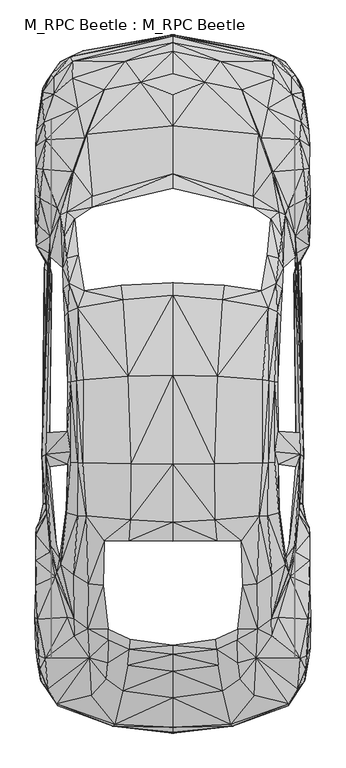
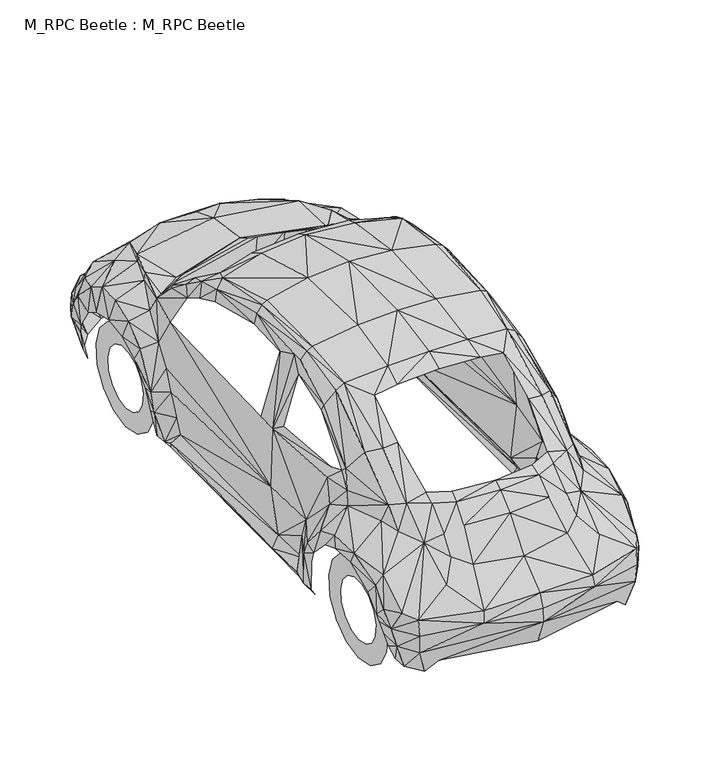
"""IFC4 building model written with IfcOpenShell, lengths in millimetres: proxy geometry, M_RPC Beetle : M_RPC Beetle."""

from ifc_helpers import new_model, si_unit, origin, place, context, project, spatial, triangles, source, transform, mapped, element, save


def m_rpc_beetle_m_rpc_beetle_aa710b07(model_context):
    return source(origin(), model_context, "Body", "Tessellation", [
        triangles([(0.0, -749.071574, 521.742899), (0.0, -720.6335569, 604.0334066), (0.0, -697.1470545, 283.3282547), (0.0, -553.0728908, 738.9057701), (0.0, -753.760096, 438.7513078), (0.0, -253.8386302, 1040.4185434), (0.0, -401.3744104, 922.0218458), (0.0, -305.0182643, 1012.9445663), (0.0, 339.5469707, 1396.6602436), (0.0, 448.9171117, 1443.1075539), (0.0, 778.6050184, 1505.0664173), (0.0, 1285.8879353, 1510.4998066), (0.0, 1742.2541199, 1403.2767002), (0.0, 2432.6093651, 967.8556761), (0.0, 3132.1224815, 632.4714237), (0.0, 3003.4724854, 772.0322365), (0.0, 2706.0784286, 929.3833151), (0.0, 3166.3445206, 220.3177475), (0.0, 2885.1195351, 859.3180424), (0.0, 3224.7104347, 396.0724085), (0.0, 3181.1549538, 556.1401817), (0.0, 3216.1220055, 530.6379956), (-338.407687, -715.988855, 523.3641664), (-331.2653541, -702.6242638, 593.8676027), (-244.8997318, -218.1706584, 1034.7659815), (-249.1500901, -276.1420835, 1003.6112698), (-257.9137267, -368.4231514, 912.4695219), (-249.2377301, 343.0524253, 1381.9373051), (-285.431542, -511.8838351, 760.9462852), (-240.2988317, 460.3974792, 1427.552108), (-236.6180971, 781.4093531, 1494.4185207), (-652.9344915, -590.6250681, 370.7455024), (-540.4532759, -593.7361427, 283.6349946), (-181.3633847, 2956.2803078, 806.8676828), (-253.3566284, 1279.4466133, 1497.179108), (-380.1225826, -444.6667534, 798.8051662), (-371.1837024, -353.5687892, 889.7717068), (-368.2478714, -222.3771967, 1004.1371098), (-368.6422151, -160.8126769, 1037.3951088), (-390.4198465, 343.0962453, 1359.9405373), (-282.758631, 1714.4295101, 1400.2533382), (-397.6060358, 87.5486986, 1216.1732225), (-463.4209139, -538.1308886, 705.2972111), (-271.6726253, 3074.4140854, 663.1441154), (-476.0843851, -323.2904411, 850.4229458), (-464.0343939, 3087.9975586, 214.4022838), (-482.5694544, 95.8303334, 1204.2108713), (-485.3738254, -159.4104914, 1005.7583771), (-569.1103566, 3073.5815781, 547.1136251), (-493.874542, 483.577278, 1392.2346416), (-583.6579788, 3101.4935371, 522.4001627), (-510.6130915, 3134.4011215, 369.6500387), (-392.1287539, 2913.6012268, 783.2935404), (-656.7905062, -598.249421, 480.4223834), (-660.6903408, -585.2354261, 576.6470695), (-562.669071, -200.2052034, 880.3069502), (-560.43436, -101.5266881, 987.8367239), (-512.8039824, 786.711355, 1449.4173431), (-542.1621832, 485.1109054, 1360.7731899), (-564.3779783, 148.6750366, 1173.0999796), (-608.8972449, -561.6174273, 218.6088221), (-511.6209151, 1259.3779255, 1457.1731197), (-542.7756269, 785.2215477, 1431.62715), (-459.1705556, 2305.6242382, 949.6711029), (-601.4481357, -92.8068715, 893.8029287), (-504.0841659, 1766.4854897, 1321.8626289), (-546.4125415, 1253.8568962, 1442.4940739), (-603.419963, 501.4988949, 1279.4466133), (-580.5468678, 789.4280497, 1379.6588104), (-607.6265013, 520.2092717, 1235.979063), (-601.6672357, 965.9276688, 1337.9439148), (-712.9653477, -503.4269022, 590.8879881), (-543.0385468, 1671.1809872, 1362.0876446), (-490.9387473, 2659.6751564, 894.1096687), (-600.0459683, 778.6050184, 1308.1913704), (-598.468521, 1244.567347, 1344.6919041), (-640.0081003, 208.2677382, 1063.2039986), (-680.8904886, -470.5194632, 218.8279221), (-538.8319722, 1968.0490585, 1181.3815962), (-581.3794115, 1249.0805889, 1402.7071129), (-644.9596149, 243.4537263, 1028.9820322), (-502.6819985, 2637.5907486, 866.5918716), (-661.1722881, 162.3463042, 955.8933249), (-690.7057325, -396.8611321, 226.9780968), (-559.5141764, 2176.4921494, 1011.8490664), (-670.6370447, 140.9630437, 873.2960409), (-662.9250154, 324.5173285, 1010.140159), (-615.5138105, 1624.5585423, 1262.9710201), (-595.0507064, 1647.2125374, 1322.1692963), (-589.8363444, 1810.8295853, 1270.2885967), (-729.3095535, -482.3065707, 373.4622334), (-752.0950087, -454.7449173, 476.8731088), (-694.5179272, 315.5346282, 958.4347395), (-727.0748062, -327.5407994, 736.0575428), (-623.3572271, 1778.4478409, 1193.6068674), (-565.035242, 2447.3759056, 934.772957), (-732.2891682, -394.1444012, 324.3420485), (-571.3888876, 2445.9300636, 884.7764448), (-699.1188091, 280.0419, 808.1822828), (-604.6907066, 1951.091518, 1171.2596123), (-587.8206971, 3015.1278786, 200.2490234), (-691.4068525, 574.6314222, 283.8102565), (-750.7366613, -381.2618663, 397.2555121), (-627.9581091, 1897.5456585, 1125.469602), (-602.8941593, 2217.067725, 949.8025629), (-619.8517725, 2074.2204849, 1075.9988571), (-710.949773, 550.0056361, 448.9171117), (-765.2404272, -360.5796985, 467.8465522), (-699.9952091, 763.1372126, 1016.187101), (-763.8382599, -313.4313409, 671.381912), (-758.3609779, -391.2085702, 565.035242), (-717.9606823, 496.6350929, 583.9646825), (-723.2188643, 461.5367266, 181.1004829), (-718.1358896, 554.8256181, 180.0050192), (-771.9884165, -342.0446016, 511.3579951), (-574.3247186, 2977.4883156, 683.0814159), (-731.2813808, 376.1351443, 185.3070212), (-541.5487032, 2807.2984131, 783.4688204), (-640.1833803, 2199.9349045, 944.8949409), (-739.4315374, 551.9336071, 222.5524585), (-782.1104731, -268.9559124, 609.6421486), (-772.8209965, -106.1275973, 756.4329706), (-722.2110043, 958.3909195, 967.6803961), (-703.8074038, 810.6798775, 292.5300731), (-725.3220789, 835.6124399, 965.0074488), (-758.2733379, 370.7893224, 225.6197313), (-785.878775, -90.0025096, 695.9639145), (-780.1824657, 80.9759712, 676.0266867), (-779.9195457, 89.5643278, 755.1622633), (-760.9024652, 444.4038334, 223.2973804), (-778.6050184, 192.2302905, 631.3321037), (-659.0690735, 2238.6700401, 850.3353058), (-771.4626492, 345.7253363, 426.4822165), (-774.7051838, 315.3593482, 502.0247349), (-781.7160931, 232.4115588, 696.3582945), (-719.7134096, 810.6360575, 185.964303), (-690.3551725, 1860.1249775, 294.1075386), (-697.1470545, 1960.2056419, 957.0763922), (-780.2701057, 377.6249516, 532.7412466), (-778.6488384, 417.28038, 440.0220151), (-746.0042467, 820.1446341, 614.0677505), (-678.173794, 2886.7845497, 671.0752447), (-698.0233818, 2078.8215122, 757.3970106), (-640.0519203, 3071.2590454, 391.9535102), (-713.4911877, 1919.5424263, 537.0792449), (-718.6617296, 1911.1731697, 193.1066541), (-705.6477711, 1983.2978371, 648.7279169), (-731.2813808, 1892.3751892, 233.5070043), (-674.4492393, 2909.8328522, 198.8030179), (-727.3815462, 2040.3052586, 190.0832013), (-722.1233643, 1974.7094078, 190.0832013), (-678.6557413, 2984.5867195, 540.8914395), (-700.0828491, 2817.5957497, 206.339749), (-696.8403145, 2993.6132034, 517.7554607), (-724.1390116, 2626.4609047, 788.1135223), (-699.5570091, 1883.7430126, 390.6389465), (-765.4157072, 2043.5477932, 362.8144094), (-742.2797647, 2459.3382568, 809.2338902), (-716.6460823, 2967.1470863, 449.8372953), (-766.9493345, 2002.4901249, 376.836228), (-732.0700682, 2726.2786491, 728.1264862), (-771.6817492, 2086.0075562, 482.5694544), (-759.6317579, 2292.960767, 780.6206657), (-769.5346418, 2144.7677776, 699.5131891), (-778.0791784, 2024.2239727, 495.1452856), (-742.9808121, 2848.794136, 602.2806793), (-782.6362404, 2187.1399006, 616.8721579), (-740.0450174, 2920.3932541, 427.6652839), (-741.6224648, 2898.4841263, 520.1654517), (-750.9119413, 2806.3345184, 398.3509395), (-782.7677004, 2314.7385075, 681.1972286), (-778.6050184, 2464.4649788, 693.9920872), (-760.4204453, 2788.5004326, 455.533641), (-774.7051838, 2684.6515388, 603.069403), (-780.8835131, 2591.1871857, 666.7810301), (-743.1122721, 809.6720901, 220.5368294), (0.0, 2350.6693085, 1011.8490664), (-459.1705556, 2241.4745201, 1007.2920044), (0.0, 1813.2394672, 1369.1424465), (-294.1513586, 1797.0267941, 1360.0720699), (-580.6345078, 850.2914858, 1382.7260651), (338.407687, -715.988855, 523.3641664), (331.2653541, -702.6242638, 593.8676027), (244.8997318, -218.1706584, 1034.7659815), (249.1500901, -276.1420835, 1003.6112698), (257.9137267, -368.4231514, 912.4695219), (249.2377301, 343.0524253, 1381.9373051), (285.431542, -511.8838351, 760.9462852), (240.2988317, 460.3974792, 1427.552108), (236.6180971, 781.4093531, 1494.4185207), (652.9344915, -590.6250681, 370.7455024), (540.4532759, -593.7361427, 283.6349946), (181.3633847, 2956.2803078, 806.8676828), (253.3566284, 1279.4466133, 1497.179108), (380.1225826, -444.6667534, 798.8051662), (371.1837024, -353.5687892, 889.7717068), (368.2478714, -222.3771967, 1004.1371098), (368.6422151, -160.8126769, 1037.3951088), (390.4198465, 343.0962453, 1359.9405373), (282.758631, 1714.4295101, 1400.2533382), (397.6060358, 87.5486986, 1216.1732225), (463.4209139, -538.1308886, 705.2972111), (271.6726253, 3074.4140854, 663.1441154), (476.0843851, -323.2904411, 850.4229458), (464.0343939, 3087.9975586, 214.4022838), (482.5694544, 95.8303334, 1204.2108713), (485.3738254, -159.4104914, 1005.7583771), (569.1103566, 3073.5815781, 547.1136251), (493.874542, 483.577278, 1392.2346416), (583.6579788, 3101.4935371, 522.4001627), (510.6130915, 3134.4011215, 369.6500387), (392.1287539, 2913.6012268, 783.2935404), (656.7905062, -598.249421, 480.4223834), (660.6903408, -585.2354261, 576.6470695), (562.669071, -200.2052034, 880.3069502), (560.43436, -101.5266881, 987.8367239), (512.8039824, 786.711355, 1449.4173431), (542.1621832, 485.1109054, 1360.7731899), (564.3779783, 148.6750366, 1173.0999796), (608.8972449, -561.6174273, 218.6088221), (511.6209151, 1259.3779255, 1457.1731197), (542.7756269, 785.2215477, 1431.62715), (459.1705556, 2305.6242382, 949.6711029), (601.4481357, -92.8068715, 893.8029287), (504.0841659, 1766.4854897, 1321.8626289), (546.4125415, 1253.8568962, 1442.4940739), (603.419963, 501.4988949, 1279.4466133), (580.5468678, 789.4280497, 1379.6588104), (607.6265013, 520.2092717, 1235.979063), (601.6672357, 965.9276688, 1337.9439148), (712.9653477, -503.4269022, 590.8879881), (543.0385468, 1671.1809872, 1362.0876446), (490.9387473, 2659.6751564, 894.1096687), (600.0459683, 778.6050184, 1308.1913704), (598.468521, 1244.567347, 1344.6919041), (640.0081003, 208.2677382, 1063.2039986), (680.9343086, -470.5194632, 218.8279221), (538.8319722, 1968.0490585, 1181.3815962), (581.3794115, 1249.0805889, 1402.7071129), (644.9596149, 243.4537263, 1028.9820322), (502.6819985, 2637.5907486, 866.5918716), (661.1722881, 162.3463042, 955.8933249), (690.7057325, -396.8611321, 226.9780968), (559.5141764, 2176.4921494, 1011.8490664), (670.6370447, 140.9630437, 873.2960409), (662.9250154, 324.5173285, 1010.140159), (615.5138105, 1624.5585423, 1262.9710201), (595.0507064, 1647.2125374, 1322.1692963), (589.8363444, 1810.8295853, 1270.2885967), (729.3095535, -482.3065707, 373.4622334), (752.0950087, -454.7449173, 476.8731088), (694.5179272, 315.5346282, 958.4347395), (727.0748062, -327.5407994, 736.0575428), (623.3572271, 1778.4478409, 1193.6068674), (565.035242, 2447.3759056, 934.772957), (732.2891682, -394.1444012, 324.3420485), (571.3888876, 2445.9300636, 884.7764448), (699.1188091, 280.0419, 808.1822828), (604.6907066, 1951.091518, 1171.2596123), (587.8206971, 3015.1278786, 200.2490234), (691.4068525, 574.6314222, 283.8102565), (750.7366613, -381.2618663, 397.2555121), (627.9581091, 1897.5456585, 1125.469602), (602.8941593, 2217.067725, 949.8025629), (619.8517725, 2074.2204849, 1075.9988571), (710.949773, 550.0056361, 448.9171117), (765.2404272, -360.5796985, 467.8465522), (699.9952091, 763.1372126, 1016.187101), (763.8382599, -313.4313409, 671.381912), (758.3609779, -391.2085702, 565.035242), (717.9606823, 496.6350929, 583.9646825), (723.2188643, 461.5367266, 181.1004829), (718.1358896, 554.8256181, 180.0050192), (771.9884165, -342.0446016, 511.3579951), (574.3247186, 2977.4883156, 683.0814159), (731.2813808, 376.1351443, 185.3070212), (541.5487032, 2807.2984131, 783.4688204), (640.1833803, 2199.9349045, 944.8949409), (739.4315374, 551.9336071, 222.5524585), (782.1104731, -268.9559124, 609.6421486), (772.8209965, -106.1275973, 756.4329706), (722.2548243, 958.3909195, 967.6803961), (703.8074038, 810.6798775, 292.5300731), (725.3220789, 835.6124399, 965.0074488), (758.2733379, 370.7893224, 225.6197313), (785.878775, -90.0025096, 695.9639145), (780.1824657, 80.9759712, 676.0266867), (779.9633657, 89.5643278, 755.1622633), (760.9024652, 444.4038334, 223.2973804), (778.6050184, 192.2302905, 631.3321037), (659.0690735, 2238.6700401, 850.3353058), (771.4626492, 345.7253363, 426.4822165), (774.7051838, 315.3593482, 502.0247349), (781.7160931, 232.4115588, 696.3582945), (719.7134096, 810.6360575, 185.964303), (690.3551725, 1860.1249775, 294.1075386), (697.1470545, 1960.2056419, 957.0763922), (780.2701057, 377.6249516, 532.7412466), (778.6488384, 417.28038, 440.0220151), (746.0042467, 820.1446341, 614.0677505), (678.173794, 2886.7845497, 671.0752447), (698.0233818, 2078.8215122, 757.3970106), (640.0519203, 3071.2590454, 391.9535102), (713.4911877, 1919.5424263, 537.0792449), (718.6617296, 1911.1731697, 193.1066541), (705.6477711, 1983.2978371, 648.7279169), (731.2813808, 1892.3751892, 233.5070043), (674.4492393, 2909.8328522, 198.8030179), (727.3815462, 2040.3052586, 190.0832013), (722.1233643, 1974.7094078, 190.0832013), (678.6557413, 2984.5867195, 540.8914395), (700.0828491, 2817.5957497, 206.339749), (696.8403145, 2993.6132034, 517.7554607), (724.1390116, 2626.4609047, 788.1135223), (699.5570091, 1883.7430126, 390.6389465), (765.4157072, 2043.5477932, 362.8144094), (742.2797647, 2459.3382568, 809.2338902), (716.6460823, 2967.1470863, 449.8372953), (766.9493345, 2002.4901249, 376.836228), (732.0700682, 2726.2786491, 728.1264862), (771.7255692, 2086.0075562, 482.5694544), (759.6317579, 2292.960767, 780.6206657), (769.5346418, 2144.7677776, 699.5131891), (778.0791784, 2024.2239727, 495.1452856), (742.9808121, 2848.794136, 602.2806793), (782.6362404, 2187.1399006, 616.8721579), (740.0450174, 2920.3932541, 427.6652839), (741.6224648, 2898.4841263, 520.1654517), (750.9119413, 2806.3345184, 398.3509395), (782.7677004, 2314.7385075, 681.1972286), (778.6050184, 2464.4649788, 693.9920872), (760.4204453, 2788.5004326, 455.533641), (774.7051838, 2684.6515388, 603.069403), (780.8835131, 2591.1871857, 666.7810301), (743.1122721, 809.6720901, 220.5368294), (459.1705556, 2241.4745201, 1007.2920044), (294.1513586, 1797.0267941, 1360.0720699), (580.6345078, 850.2914858, 1382.7260651), (-693.6415998, 2431.9082451, 0.0015117), (-693.6415998, 2431.9082451, 117.9161946), (-693.6415998, 2558.849334, 26.9935013), (-693.6415998, 2509.4663017, 134.3918241), (-693.6415998, 2663.794091, 103.2371124), (-693.6415998, 2573.6600578, 181.0143508), (-693.6415998, 2728.6886765, 215.6307153), (-693.6415998, 2613.3154861, 249.7212399), (-693.6415998, 2742.2721497, 344.6752187), (-693.6415998, 2621.5969574, 328.5939328), (-693.6415998, 2702.1786667, 468.1109982), (-693.6415998, 2597.102813, 404.0049911), (-693.6415998, 2615.3310608, 564.5109644), (-693.6415998, 2544.0389008, 462.94042), (-693.6415998, 2496.8028305, 617.3118113), (-693.6415998, 2471.5636734, 495.2344153), (-693.6415998, 2367.0135143, 617.3118113), (-693.6415998, 2392.2528168, 495.2344153), (-693.6415998, 2248.4854294, 564.5109644), (-693.6415998, 2319.7775894, 462.94042), (-693.6415998, 2161.6378235, 468.1109982), (-693.6415998, 2266.7136772, 404.0049911), (-693.6415998, 2121.5441952, 344.6752187), (-693.6415998, 2242.2193874, 328.5939328), (-693.6415998, 2135.1278137, 215.6307153), (-693.6415998, 2250.501004, 249.7212399), (-693.6415998, 2200.0225445, 103.2371124), (-693.6415998, 2290.1564323, 181.0143508), (-693.6415998, 2304.9670109, 26.9935013), (-693.6415998, 2354.3500431, 134.3918241), (693.6415998, 2431.9082451, 0.0015117), (693.6415998, 2431.9082451, 117.9161946), (693.6415998, 2304.9670109, 26.9935013), (693.6415998, 2354.3500431, 134.3918241), (693.6415998, 2200.0225445, 103.2371124), (693.6415998, 2290.1564323, 181.0143508), (693.6415998, 2135.1278137, 215.6307153), (693.6415998, 2250.501004, 249.7212399), (693.6415998, 2121.5441952, 344.6752187), (693.6415998, 2242.2193874, 328.5939328), (693.6415998, 2161.6378235, 468.1109982), (693.6415998, 2266.7136772, 404.0049911), (693.6415998, 2248.4854294, 564.5109644), (693.6415998, 2319.7775894, 462.94042), (693.6415998, 2367.0135143, 617.3118113), (693.6415998, 2392.2528168, 495.2344153), (693.6415998, 2496.8028305, 617.3118113), (693.6415998, 2471.5636734, 495.2344153), (693.6415998, 2615.3310608, 564.5109644), (693.6415998, 2544.0389008, 462.94042), (693.6415998, 2702.1786667, 468.1109982), (693.6415998, 2597.102813, 404.0049911), (693.6415998, 2742.2721497, 344.6752187), (693.6415998, 2621.5969574, 328.5939328), (693.6415998, 2728.6886765, 215.6307153), (693.6415998, 2613.3154861, 249.7212399), (693.6415998, 2663.794091, 103.2371124), (693.6415998, 2573.6600578, 181.0143508), (693.6415998, 2558.849334, 26.9935013), (693.6415998, 2509.4663017, 134.3918241), (-693.6415998, -13.583631, 0.0015117), (-693.6415998, -13.583631, 117.9161946), (-693.6415998, 113.3575975, 26.9935013), (-693.6415998, 63.9745244, 134.3918241), (-693.6415998, 218.3021002, 103.2371124), (-693.6415998, 128.1681397, 181.0143508), (-693.6415998, 283.1968128, 215.6307153), (-693.6415998, 167.823568, 249.7212399), (-693.6415998, 296.7804314, 344.6752187), (-693.6415998, 176.1052028, 328.5939328), (-693.6415998, 256.6868212, 468.1109982), (-693.6415998, 151.6108585, 404.0049911), (-693.6415998, 169.8392153, 564.5109644), (-693.6415998, 98.5470553, 462.94042), (-693.6415998, 51.3110713, 617.3118113), (-693.6415998, 26.0718098, 495.2344153), (-693.6415998, -78.4783311, 617.3118113), (-693.6415998, -53.2390741, 495.2344153), (-693.6415998, -197.0064706, 564.5109644), (-693.6415998, -125.7143196, 462.94042), (-693.6415998, -283.8540765, 468.1109982), (-693.6415998, -178.7781137, 404.0049911), (-693.6415998, -323.9477048, 344.6752187), (-693.6415998, -203.2724762, 328.5939328), (-693.6415998, -310.3640862, 215.6307153), (-693.6415998, -194.9908414, 249.7212399), (-693.6415998, -245.4693737, 103.2371124), (-693.6415998, -155.335395, 181.0143508), (-693.6415998, -140.5248618, 26.9935013), (-693.6415998, -91.1417842, 134.3918241), (693.6415998, -13.583631, 0.0015117), (693.6415998, -13.583631, 117.9161946), (693.6415998, -140.5248618, 26.9935013), (693.6415998, -91.1417842, 134.3918241), (693.6415998, -245.4693737, 103.2371124), (693.6415998, -155.335395, 181.0143508), (693.6415998, -310.3640862, 215.6307153), (693.6415998, -194.9908414, 249.7212399), (693.6415998, -323.9477048, 344.6752187), (693.6415998, -203.2724762, 328.5939328), (693.6415998, -283.8540765, 468.1109982), (693.6415998, -178.7781137, 404.0049911), (693.6415998, -197.0064706, 564.5109644), (693.6415998, -125.7143196, 462.94042), (693.6415998, -78.4783311, 617.3118113), (693.6415998, -53.2390741, 495.2344153), (693.6415998, 51.3110713, 617.3118113), (693.6415998, 26.0718098, 495.2344153), (693.6415998, 169.8392153, 564.5109644), (693.6415998, 98.5470553, 462.94042), (693.6415998, 256.6868212, 468.1109982), (693.6415998, 151.6108585, 404.0049911), (693.6415998, 296.7804314, 344.6752187), (693.6415998, 176.1052028, 328.5939328), (693.6415998, 283.1968128, 215.6307153), (693.6415998, 167.823568, 249.7212399), (693.6415998, 218.3021002, 103.2371124), (693.6415998, 128.1681397, 181.0143508), (693.6415998, 113.3575975, 26.9935013), (693.6415998, 63.9745244, 134.3918241)], [[67, 58, 62], [67, 63, 58], [53, 82, 74], [34, 17, 19], [118, 82, 53], [155, 98, 82], [155, 158, 98], [34, 74, 17], [172, 155, 175], [172, 158, 155], [159, 168, 169], [166, 142, 169], [175, 161, 174], [175, 155, 161], [142, 152, 169], [154, 169, 152], [160, 145, 165], [160, 156, 145], [162, 160, 165], [162, 157, 160], [34, 53, 74], [74, 96, 64], [82, 96, 74], [82, 98, 96], [36, 29, 27], [29, 43, 24], [23, 55, 54], [23, 24, 55], [23, 2, 24], [23, 1, 2], [5, 1, 23], [134, 140, 133], [134, 139, 140], [117, 130, 113], [117, 126, 130], [113, 120, 114], [113, 130, 120], [140, 112, 107], [140, 139, 112], [92, 108, 103], [91, 103, 97], [91, 92, 103], [61, 33, 32], [84, 78, 91], [84, 91, 97], [38, 26, 25], [77, 81, 83], [63, 50, 58], [63, 59, 50], [68, 63, 69], [68, 59, 63], [181, 75, 69], [74, 64, 17], [64, 14, 17], [64, 178, 14], [178, 177, 14], [34, 19, 16], [53, 34, 44], [21, 44, 15], [21, 49, 44], [44, 34, 15], [34, 16, 15], [22, 49, 21], [22, 51, 49], [20, 51, 22], [20, 52, 51], [18, 52, 20], [18, 46, 52], [51, 152, 49], [51, 154, 152], [101, 144, 46], [144, 52, 46], [101, 159, 144], [159, 169, 154], [101, 168, 159], [101, 149, 168], [149, 170, 168], [149, 153, 170], [168, 173, 169], [168, 170, 173], [49, 142, 116], [49, 152, 142], [49, 116, 44], [116, 142, 118], [161, 155, 118], [155, 82, 118], [142, 161, 118], [158, 132, 98], [158, 163, 132], [172, 163, 158], [172, 171, 163], [98, 119, 96], [98, 132, 119], [171, 164, 163], [171, 167, 164], [163, 143, 132], [163, 164, 143], [96, 105, 64], [96, 119, 105], [105, 178, 64], [105, 85, 178], [167, 165, 164], [167, 162, 165], [165, 143, 164], [165, 147, 143], [150, 160, 157], [150, 151, 160], [151, 156, 160], [151, 148, 137], [13, 35, 12], [13, 41, 35], [12, 31, 11], [12, 35, 31], [35, 58, 31], [35, 62, 58], [11, 30, 10], [11, 31, 30], [31, 50, 30], [31, 58, 50], [10, 28, 9], [10, 30, 28], [30, 40, 28], [30, 50, 40], [125, 75, 181], [125, 109, 75], [125, 87, 109], [125, 93, 87], [123, 141, 125], [137, 141, 156], [137, 124, 141], [148, 124, 137], [148, 176, 124], [146, 176, 148], [146, 136, 176], [141, 112, 125], [112, 93, 125], [112, 99, 93], [124, 112, 141], [124, 107, 112], [124, 102, 107], [176, 102, 124], [176, 120, 102], [136, 120, 176], [136, 114, 120], [47, 40, 50], [47, 42, 40], [48, 42, 47], [48, 39, 42], [57, 47, 60], [57, 48, 47], [60, 50, 59], [60, 47, 50], [59, 77, 60], [59, 68, 77], [77, 57, 60], [77, 83, 57], [70, 77, 68], [70, 81, 77], [75, 68, 69], [75, 70, 68], [26, 6, 25], [26, 8, 6], [27, 8, 26], [27, 7, 8], [29, 7, 27], [29, 4, 7], [24, 4, 29], [24, 2, 4], [32, 5, 23], [33, 5, 32], [33, 3, 5], [32, 23, 54], [55, 45, 72], [55, 24, 43], [99, 83, 93], [99, 86, 83], [135, 86, 99], [135, 129, 86], [131, 129, 135], [131, 128, 129], [93, 81, 87], [93, 83, 81], [128, 122, 129], [128, 127, 122], [122, 86, 129], [122, 65, 86], [86, 57, 83], [86, 65, 57], [127, 110, 122], [127, 121, 110], [110, 94, 122], [122, 94, 65], [94, 56, 65], [56, 57, 65], [56, 48, 57], [56, 45, 48], [94, 45, 56], [115, 110, 121], [115, 111, 110], [111, 94, 110], [111, 72, 94], [108, 92, 115], [92, 111, 115], [78, 32, 91], [78, 61, 32], [45, 38, 48], [45, 37, 38], [37, 26, 38], [37, 27, 26], [36, 27, 37], [134, 135, 139], [134, 131, 135], [139, 99, 112], [139, 135, 99], [126, 140, 130], [126, 133, 140], [130, 107, 120], [130, 140, 107], [120, 107, 102], [45, 36, 37], [92, 55, 72], [92, 54, 55], [91, 54, 92], [91, 32, 54], [92, 72, 111], [72, 45, 94], [43, 45, 55], [43, 36, 45], [43, 29, 36], [79, 90, 66], [79, 100, 90], [90, 73, 66], [85, 100, 79], [85, 106, 100], [85, 105, 106], [105, 119, 106], [95, 88, 89], [90, 89, 73], [89, 67, 73], [73, 67, 62], [89, 76, 80], [89, 80, 67], [88, 76, 89], [73, 35, 41], [73, 62, 35], [69, 63, 181], [80, 63, 67], [76, 71, 80], [146, 148, 151], [141, 147, 145], [151, 137, 156], [173, 166, 169], [173, 174, 166], [166, 174, 161], [166, 161, 142], [52, 144, 51], [144, 154, 51], [144, 159, 154], [116, 53, 44], [116, 118, 53], [119, 143, 138], [143, 119, 132], [143, 147, 138], [138, 104, 119], [119, 104, 106], [104, 100, 106], [104, 90, 100], [104, 95, 90], [95, 89, 90], [25, 39, 38], [38, 39, 48], [141, 138, 147], [156, 141, 145], [165, 145, 147], [41, 179, 180], [41, 13, 179], [66, 41, 180], [66, 73, 41], [123, 125, 71], [125, 181, 71], [71, 181, 80], [181, 63, 80], [138, 141, 123], [226, 221, 217], [226, 217, 222], [212, 233, 241], [193, 19, 17], [277, 212, 241], [314, 241, 257], [314, 257, 317], [193, 17, 233], [331, 334, 314], [331, 314, 317], [318, 328, 327], [325, 328, 301], [334, 333, 320], [334, 320, 314], [301, 328, 311], [313, 311, 328], [319, 324, 304], [319, 304, 315], [321, 324, 319], [321, 319, 316], [193, 233, 212], [233, 223, 255], [241, 233, 255], [241, 255, 257], [195, 186, 188], [188, 183, 202], [182, 213, 214], [182, 214, 183], [182, 183, 2], [182, 2, 1], [5, 182, 1], [293, 292, 299], [293, 299, 298], [276, 272, 289], [276, 289, 285], [272, 273, 279], [272, 279, 289], [299, 266, 271], [299, 271, 298], [251, 262, 267], [250, 256, 262], [250, 262, 251], [220, 191, 192], [243, 250, 237], [243, 256, 250], [197, 184, 185], [236, 242, 240], [222, 217, 209], [222, 209, 218], [227, 228, 222], [227, 222, 218], [338, 228, 234], [233, 17, 223], [223, 17, 14], [223, 14, 336], [336, 14, 177], [193, 16, 19], [212, 203, 193], [21, 15, 203], [21, 203, 208], [203, 15, 193], [193, 15, 16], [22, 21, 208], [22, 208, 210], [20, 22, 210], [20, 210, 211], [18, 20, 211], [18, 211, 205], [210, 208, 311], [210, 311, 313], [260, 205, 303], [303, 205, 211], [260, 303, 318], [318, 313, 328], [260, 318, 327], [260, 327, 308], [308, 327, 329], [308, 329, 312], [327, 328, 332], [327, 332, 329], [208, 275, 301], [208, 301, 311], [208, 203, 275], [275, 277, 301], [320, 277, 314], [314, 277, 241], [301, 277, 320], [317, 257, 291], [317, 291, 322], [331, 317, 322], [331, 322, 330], [257, 255, 278], [257, 278, 291], [330, 322, 323], [330, 323, 326], [322, 291, 302], [322, 302, 323], [255, 223, 264], [255, 264, 278], [264, 223, 336], [264, 336, 244], [326, 323, 324], [326, 324, 321], [324, 323, 302], [324, 302, 306], [309, 316, 319], [309, 319, 310], [310, 319, 315], [310, 296, 307], [13, 12, 194], [13, 194, 200], [12, 11, 190], [12, 190, 194], [194, 190, 217], [194, 217, 221], [11, 10, 189], [11, 189, 190], [190, 189, 209], [190, 209, 217], [10, 9, 187], [10, 187, 189], [189, 187, 199], [189, 199, 209], [284, 338, 234], [284, 234, 268], [284, 268, 246], [284, 246, 252], [282, 284, 300], [296, 315, 300], [296, 300, 283], [307, 296, 283], [307, 283, 335], [305, 307, 335], [305, 335, 295], [300, 284, 271], [271, 284, 252], [271, 252, 258], [283, 300, 271], [283, 271, 266], [283, 266, 261], [335, 283, 261], [335, 261, 279], [295, 335, 279], [295, 279, 273], [206, 209, 199], [206, 199, 201], [207, 206, 201], [207, 201, 198], [216, 219, 206], [216, 206, 207], [219, 218, 209], [219, 209, 206], [218, 219, 236], [218, 236, 227], [236, 219, 216], [236, 216, 242], [229, 227, 236], [229, 236, 240], [234, 228, 227], [234, 227, 229], [185, 184, 6], [185, 6, 8], [186, 185, 8], [186, 8, 7], [188, 186, 7], [188, 7, 4], [183, 188, 4], [183, 4, 2], [191, 182, 5], [192, 191, 5], [192, 5, 3], [191, 213, 182], [214, 231, 204], [214, 202, 183], [258, 252, 242], [258, 242, 245], [294, 258, 245], [294, 245, 288], [290, 294, 288], [290, 288, 287], [252, 246, 240], [252, 240, 242], [287, 288, 281], [287, 281, 286], [281, 288, 245], [281, 245, 224], [245, 242, 216], [245, 216, 224], [286, 281, 269], [286, 269, 280], [269, 281, 253], [281, 224, 253], [253, 224, 215], [215, 224, 216], [215, 216, 207], [215, 207, 204], [253, 215, 204], [274, 280, 269], [274, 269, 270], [270, 269, 253], [270, 253, 231], [267, 274, 251], [251, 274, 270], [237, 250, 191], [237, 191, 220], [204, 207, 197], [204, 197, 196], [196, 197, 185], [196, 185, 186], [195, 196, 186], [293, 298, 294], [293, 294, 290], [298, 271, 258], [298, 258, 294], [285, 289, 299], [285, 299, 292], [289, 279, 266], [289, 266, 299], [279, 261, 266], [204, 196, 195], [251, 231, 214], [251, 214, 213], [250, 251, 213], [250, 213, 191], [251, 270, 231], [231, 253, 204], [202, 214, 204], [202, 204, 195], [202, 195, 188], [238, 225, 249], [238, 249, 259], [249, 225, 232], [244, 238, 259], [244, 259, 265], [244, 265, 264], [264, 265, 278], [254, 248, 247], [249, 232, 248], [248, 232, 226], [232, 221, 226], [248, 239, 235], [248, 226, 239], [247, 248, 235], [232, 200, 194], [232, 194, 221], [228, 338, 222], [239, 226, 222], [235, 239, 230], [305, 310, 307], [300, 304, 306], [310, 315, 296], [332, 328, 325], [332, 325, 333], [325, 320, 333], [325, 301, 320], [211, 210, 303], [303, 210, 313], [303, 313, 318], [275, 203, 212], [275, 212, 277], [278, 297, 302], [302, 291, 278], [302, 297, 306], [297, 278, 263], [278, 265, 263], [263, 265, 259], [263, 259, 249], [263, 249, 254], [254, 249, 248], [184, 197, 198], [197, 207, 198], [300, 306, 297], [315, 304, 300], [324, 306, 304], [200, 337, 179], [200, 179, 13], [225, 337, 200], [225, 200, 232], [282, 230, 284], [284, 230, 338], [230, 239, 338], [338, 239, 222], [297, 282, 300], [339, 342, 341], [339, 340, 342], [341, 344, 343], [341, 342, 344], [343, 346, 345], [343, 344, 346], [345, 348, 347], [345, 346, 348], [347, 350, 349], [347, 348, 350], [349, 352, 351], [349, 350, 352], [351, 354, 353], [351, 352, 354], [353, 356, 355], [353, 354, 356], [355, 358, 357], [355, 356, 358], [357, 360, 359], [357, 358, 360], [359, 362, 361], [359, 360, 362], [361, 364, 363], [361, 362, 364], [363, 366, 365], [363, 364, 366], [365, 368, 367], [365, 366, 368], [367, 340, 339], [367, 368, 340], [369, 372, 371], [369, 370, 372], [371, 374, 373], [371, 372, 374], [373, 376, 375], [373, 374, 376], [375, 378, 377], [375, 376, 378], [377, 380, 379], [377, 378, 380], [379, 382, 381], [379, 380, 382], [381, 384, 383], [381, 382, 384], [383, 386, 385], [383, 384, 386], [385, 388, 387], [385, 386, 388], [387, 390, 389], [387, 388, 390], [389, 392, 391], [389, 390, 392], [391, 394, 393], [391, 392, 394], [393, 396, 395], [393, 394, 396], [395, 398, 397], [395, 396, 398], [397, 370, 369], [397, 398, 370], [399, 402, 401], [399, 400, 402], [401, 404, 403], [401, 402, 404], [403, 406, 405], [403, 404, 406], [405, 408, 407], [405, 406, 408], [407, 410, 409], [407, 408, 410], [409, 412, 411], [409, 410, 412], [411, 414, 413], [411, 412, 414], [413, 416, 415], [413, 414, 416], [415, 418, 417], [415, 416, 418], [417, 420, 419], [417, 418, 420], [419, 422, 421], [419, 420, 422], [421, 424, 423], [421, 422, 424], [423, 426, 425], [423, 424, 426], [425, 428, 427], [425, 426, 428], [427, 400, 399], [427, 428, 400], [429, 432, 431], [429, 430, 432], [431, 434, 433], [431, 432, 434], [433, 436, 435], [433, 434, 436], [435, 438, 437], [435, 436, 438], [437, 440, 439], [437, 438, 440], [439, 442, 441], [439, 440, 442], [441, 444, 443], [441, 442, 444], [443, 446, 445], [443, 444, 446], [445, 448, 447], [445, 446, 448], [447, 450, 449], [447, 448, 450], [449, 452, 451], [449, 450, 452], [451, 454, 453], [451, 452, 454], [453, 456, 455], [453, 454, 456], [455, 458, 457], [455, 456, 458], [457, 430, 429], [457, 458, 430]], closed=False),
    ])


if __name__ == "__main__":
    model = new_model("IFC4")
    model_context = context("Model", 3, world=origin())
    ifc_project = project(units=[si_unit("LENGTHUNIT", "METRE", prefix="MILLI")], contexts=[model_context])
    site = spatial("IfcSite", under=ifc_project)
    building = spatial("IfcBuilding", under=site)
    placement = place(None, origin())
    m_rpc_beetle_m_rpc_beetle_shape = m_rpc_beetle_m_rpc_beetle_aa710b07(model_context)
    element("IfcBuildingElementProxy", 1, Name="M_RPC Beetle : M_RPC Beetle", ObjectType="M_RPC Beetle : M_RPC Beetle", at=placement, inside=building, context=model_context, shape_type="MappedRepresentation", body=[
        mapped(m_rpc_beetle_m_rpc_beetle_shape, transform((0.0, 0.0, 0.0), x_axis=(1.0, 0.0, 0.0), y_axis=(0.0, 1.0, 0.0), z_axis=(0.0, 0.0, 1.0))),
    ])
    save(model, "model.ifc")

# Revit data of these elements
# Type "M_RPC Beetle : M_RPC Beetle"
#   built-in parameter 1005198 = "{2, 15},{39, RPC-16-0U6E-L4EG-ENH1-J3KF-SVEL-0TX4-C0},{1, 0},{1, 0},{2, 45},{1, 8},{5, Color},{1, 0},{1, 0},{3, 0.8},{3, 0.8},{3, 0.8},{1, 8},{7, BBoxMin},{1, 0},{1, 0},{1, 0},{1, 0},{1, 0},{1, 8},{7, BBoxMax},{1, 0},{1, 0},{1, 0},{1, 0},{1, 0},{2, 11},{9, RPCTypeId},{1, 0},{1, 0},{39, RPC-16-0U6E-L4EG-ENH1-J3KF-SVEL-0TX4-C0},{1, 6},{14, RPCPlantHeight},{1, 0},{1, 0},{4, 4.92},{2, 11},{7, keyword},{1, 0},{1, 0},{27, :Geometry:RPC:VW Beetle [4]},{2, 11},{8, category},{1, 0},{1, 0},{21, :Auto_Economy/Midsize},{2, 11},{12, LocalizedUID},{1, 0},{1, 0},{13, VW Beetle [4]},{2, 14},{6, Height},{1, 0},{1, 0},{4, 4.92},{1, 2},{16, Cast Reflections},{1, 0},{1, 0},{1, 0},{1, 4},{12, Transparency},{1, 0},{1, 0},{2, 18},{1, 4},{7, Tinting},{1, 0},{1, 0},{2, 50},{1, 2},{11, Use Tinting},{1, 0},{1, 0},{1, 0},{1, 2},{13, License Plate},{1, 0},{1, 0},{1, 0},{2, 11},{21, License Plate Texture},{1, 0},{1, 0},{64, __RPC:/object data/textures/car/plate/textures/default/rgb/0/0/0},{2, 11},{23, i_License Plate Texture},{1, 0},{1, 0},{0, },{1, 2},{12, Custom Plate},{1, 0},{1, 0},{1, 0},{2, 11},{23, License Plate File Name},{1, 0},{1, 0},{0, },{2, 11},{20, AdvancedUIDefinition},{1, 0},{1, 0},{0, },{2, 11},{10, AssetLibID},{1, 0},{1, 0},{36, 4D3F6E72-3F99-4203-98E9-AF80B3C7A7A4},{2, 11},{10, BaseSchema},{1, 0},{1, 0},{9, RPCSchema},{2, 11},{12, ExchangeGUID},{1, 0},{1, 0},{0, },{1, 2},{6, Hidden},{1, 0},{1, 0},{1, 0},{1, 4},{11, RPCCategory},{1, 0},{1, 0},{1, 0},{2, 11},{8, RPCImage},{1, 0},{1, 0},{0, },{1, 4},{13, SchemaVersion},{1, 0},{1, 0},{1, 4},{2, 11},{12, UIDefinition},{1, 0},{1, 0},{0, },{2, 11},{6, UIName},{1, 0},{1, 0},{39, RPC-16-0U6E-L4EG-ENH1-J3KF-SVEL-0TX4-C0},{2, 11},{11, VersionGUID},{1, 0},{1, 0},{9, RPCSchema},{2, 11},{9, assettype},{1, 0},{1, 0},{11, RPCGeometry},{2, 11},{11, description},{1, 0},{1, 0},{0, },{2, 11},{9, localname},{1, 0},{1, 0},{3, RPC},{2, 11},{9, localtype},{1, 0},{1, 0},{3, RPC},{1, 4},{8, revision},{1, 0},{1, 0},{1, 1},{2, 11},{9, thumbnail},{1, 0},{1, 0},{0, },{1, 4},{7, version},{1, 0},{1, 0},{1, 1},{1, 2},{20, RPC_Cast Reflections},{1, 0},{1, 0},{1, 0},{1, 4},{16, RPC_Transparency},{1, 0},{1, 0},{2, 10},{1, 4},{11, RPC_Tinting},{1, 0},{1, 0},{2, 30},{1, 2},{15, RPC_Use Tinting},{1, 0},{1, 0},{1, 0},{1, 2},{17, RPC_License Plate},{1, 0},{1, 0},{1, 0},{2, 11},{25, RPC_License Plate Texture},{1, 0},{1, 0},{64, __RPC:/object data/textures/car/plate/textures/default/rgb/0/0/0},{2, 11},{27, RPC_i_License Plate Texture},{1, 0},{1, 0},{0, },{1, 2},{16, RPC_Custom Plate},{1, 0},{1, 0},{1, 0},{2, 11},{27, RPC_License Plate File Name},{1, 0},{1, 0},{0, },{21, assetlibrary_base.fbx},{1, 5},"
#   built-in parameter 1005195 = "RPC-16-0U6E-L4EG-ENH1-J3KF-SVEL-0TX4-C0"
#   Height = 0
